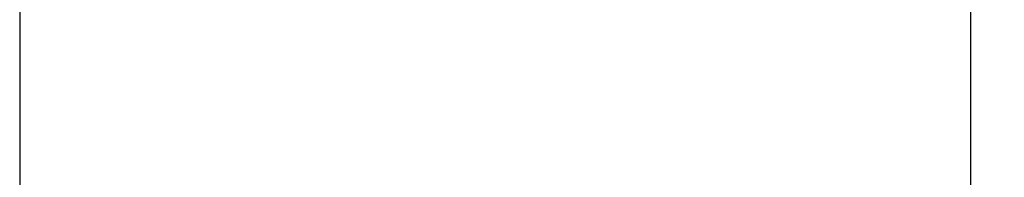
# Model space of a CAD drawing. Units: inches. Extents: x 2091 to 2899, y 967 to 2217.
# Tile 4 of 256: x 2212 to 2312, y 1065 to 1081. Entities that reach past the tile are written whole.
import ezdxf

# ---------------------------------------------------------------- set-up
doc = ezdxf.new("R2010")
doc.units = ezdxf.units.IN
doc.layers.add('A-ANNO-DIMS', color=2, linetype='Continuous', lineweight=18)
doc.styles.get("Standard").update_dxf_attribs({"font": 'arial.ttf'})
doc.dimstyles.new('ISO-25', dxfattribs={"dimtxt": 4, "dimasz": 4, "dimexe": 1.25, "dimexo": 0.625, "dimtad": 1, "dimdec": 0, "dimlunit": 3, "dimtxsty": 'Standard', "dimcen": 2.5, "dimadec": 0, "dimazin": 0, "dimtfac": 1, "dimtdec": 0, "dimtmove": 0, "dimatfit": 3, "dimfxl": 1, "dimarcsym": 0})

# ---------------------------------------------------------------- blocks, each defined once
blk = doc.blocks.new('*D71')
at = {"layer": 'A-ANNO-DIMS', "color": 0, "lineweight": -2, "transparency": 16777216}
for p, q in [((2212.144, 1351.294), (2212.144, 969.464)), ((2452.144, 1351.294), (2452.144, 969.464)), ((2216.144, 970.714), (2448.144, 970.714))]:
    blk.add_line(p, q, dxfattribs=at)
at = {"layer": 'A-ANNO-DIMS', "color": 0, "transparency": 16777216}
for points in [[(2216.144, 971.381), (2216.144, 970.048), (2212.144, 970.714)], [(2448.144, 971.381), (2448.144, 970.048), (2452.144, 970.714)]]:
    blk.add_solid(points, dxfattribs=at)
at = {"layer": 'Defpoints', "color": 0, "transparency": 16777216}
for p in [(2212.144, 1351.919), (2452.144, 1351.919), (2452.144, 970.714)]:
    blk.add_point(p, dxfattribs=at)
at = {"layer": 'A-ANNO-DIMS', "color": 0, "transparency": 16777216, "insert": (2332.144, 973.382), "char_height": 4, "attachment_point": 5}
blk.add_mtext('20\'-0"', dxfattribs=at)
blk = doc.blocks.new('*D75')
at = {"layer": 'A-ANNO-DIMS', "color": 0, "lineweight": -2, "transparency": 16777216}
for p, q in [((2212.144, 1274.794), (2212.144, 969.464)), ((2308.144, 1274.794), (2308.144, 969.464)), ((2216.144, 970.714), (2304.144, 970.714))]:
    blk.add_line(p, q, dxfattribs=at)
at = {"layer": 'A-ANNO-DIMS', "color": 0, "transparency": 16777216}
for points in [[(2216.144, 971.381), (2216.144, 970.048), (2212.144, 970.714)], [(2304.144, 971.381), (2304.144, 970.048), (2308.144, 970.714)]]:
    blk.add_solid(points, dxfattribs=at)
at = {"layer": 'Defpoints', "color": 0, "transparency": 16777216}
for p in [(2212.144, 1275.419), (2308.144, 1275.419), (2308.144, 970.714)]:
    blk.add_point(p, dxfattribs=at)
at = {"layer": 'A-ANNO-DIMS', "color": 0, "transparency": 16777216, "insert": (2260.144, 973.382), "char_height": 4, "attachment_point": 5}
blk.add_mtext('8\'-0"', dxfattribs=at)

msp = doc.modelspace()

# ---------------------------------------------------------------- dimensions: what is measured, and where the dimension line sits
at = {"layer": 'A-ANNO-DIMS'}
for base, p1, p2, picture, middle in [((2452.144, 970.714), (2212.144, 1351.919), (2452.144, 1351.919), '*D71', (2332.144, 973.382)), ((2308.144, 970.714), (2212.144, 1275.419), (2308.144, 1275.419), '*D75', (2260.144, 973.382))]:
    dim = msp.add_linear_dim(base=base, p1=p1, p2=p2, dimstyle='ISO-25', override={"dimdec": 1, "dimlfac": 1, "dimrnd": 0, "dimzin": 1, "dimdsep": 46, "dimlunit": 4, "dimfrac": 2}, dxfattribs=at)
    dim.commit()
    dim.dimension.update_dxf_attribs({"geometry": picture, "text_midpoint": middle})

doc.saveas('drawing.dxf')
